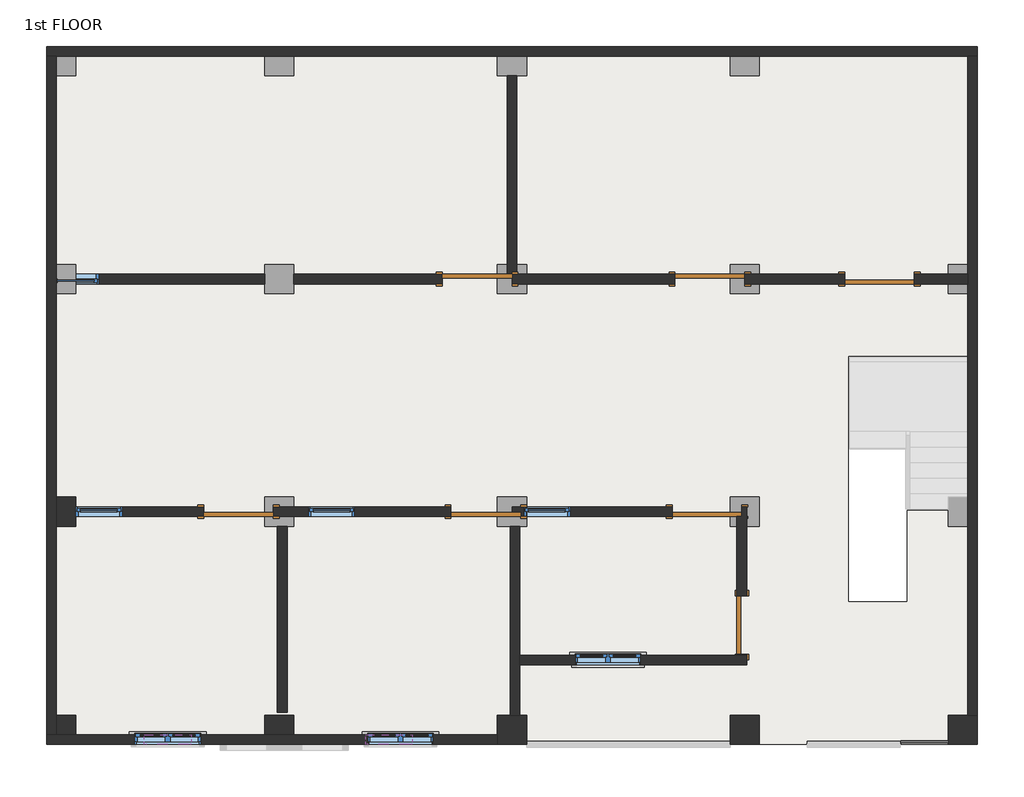
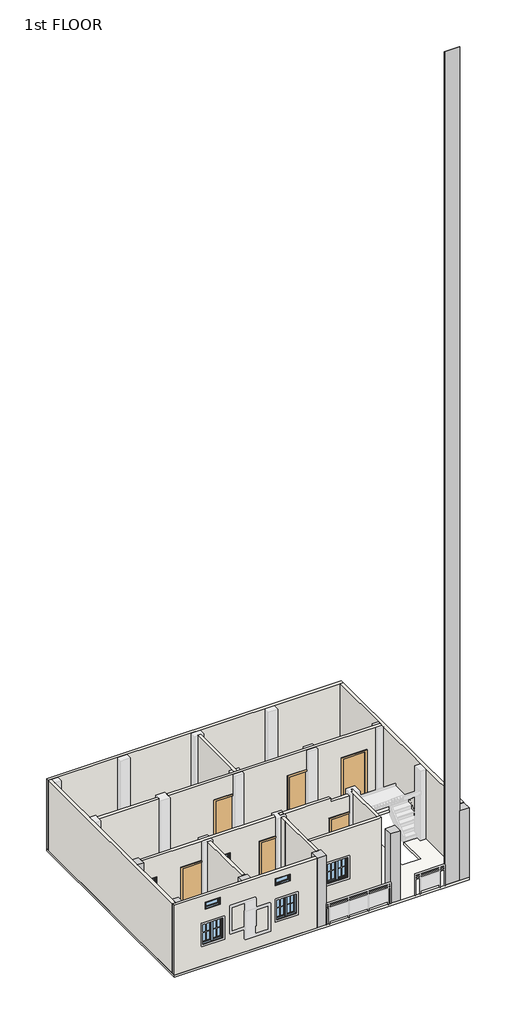
# One storey, part 1 of 2: 15 walls, 9 windows, 7 doors, 6 columns, 1 plate, 1 slab.
"""IFC4 building model written with IfcOpenShell, lengths in millimetres."""

from ifc_helpers import new_model, si_unit, frame, origin, place, context, project, spatial, polyline, outline, extrude, faceted_brep, transform, mapped, element, save
from components import door_e00f436c, door_a1797ceb, system_panel_glazed_6238d1ea, window_4c2727af, window_0bf3737e, window_78893e6c, window_0d9958e7

model = new_model("IFC4")

# Units and contexts
model_context = context("Model", 3, world=origin())
ifc_project = project(units=[si_unit("LENGTHUNIT", "METRE", prefix="MILLI")], contexts=[model_context])

# Site, building, storey
site = spatial("IfcSite", under=ifc_project)
building = spatial("IfcBuilding", under=site)
storey = spatial("IfcBuildingStorey", under=building, Name="1st FLOOR", Elevation=3048.0)

# Columns
placement = place(None, origin())
element("IfcColumn", 1, ObjectType="column family : column family", at=placement, inside=storey, context=model_context, shape_type="SweptSolid", body=[
    extrude(outline(polyline([(-15433.597125, 2867.2065522), (-15433.597125, 2486.2065522), (-15687.597125, 2486.2065522), (-15687.597125, 2867.2065522), (-15433.597125, 2867.2065522)])), frame((0.0, 0.0, 3053.0), z_axis=(0.0, 0.0, 1.0), x_axis=(1.0, 0.0, 0.0)), (0.0, 0.0, 1.0), 3038.0),
])
element("IfcColumn", 2, ObjectType="column family : column family", at=placement, inside=storey, context=model_context, shape_type="Brep", body=[
    faceted_brep([(-15433.597125, 9.7065522, 3053.0), (-15433.597125, -244.2934478, 3053.0), (-15687.597125, -244.2934478, 3053.0), (-15687.597125, 9.7065522, 3053.0), (-15433.597125, 9.7065522, 6091.0), (-15433.597125, -244.2934478, 6091.0), (-15687.597125, 9.7065522, 6091.0), (-15687.597125, -244.2934478, 6091.0), (-15687.597125, -244.2934478, 5943.6)], [[[0, 1, 2, 3]], [[0, 4, 5, 1]], [[4, 0, 3, 6]], [[5, 4, 6, 7]], [[1, 5, 7, 8, 2]], [[3, 2, 8, 7, 6]]]),
])
element("IfcColumn", 3, ObjectType="column family : column family", at=placement, inside=storey, context=model_context, shape_type="Brep", body=[
    faceted_brep([(-3622.597125, 9.7065522, 3053.0), (-3622.597125, -371.2934478, 3053.0), (-4003.597125, -371.2934478, 3053.0), (-4003.597125, 9.7065522, 3053.0), (-3622.597125, 9.7065522, 6091.0), (-3622.597125, -371.2934478, 6091.0), (-3622.597125, 9.7065522, 5943.6), (-4003.597125, -371.2934478, 6091.0), (-4003.597125, 9.7065522, 6091.0)], [[[0, 1, 2, 3]], [[4, 5, 1, 0, 6]], [[5, 7, 2, 1]], [[7, 8, 3, 2]], [[8, 4, 6, 0, 3]], [[4, 8, 7, 5]]]),
])
element("IfcColumn", 4, ObjectType="column family : column family", at=placement, inside=storey, context=model_context, shape_type="SweptSolid", body=[
    extrude(outline(polyline([(-6480.097125, 9.7065522), (-6480.097125, -371.2934478), (-6861.097125, -371.2934478), (-6861.097125, 9.7065522), (-6480.097125, 9.7065522)])), frame((0.0, 0.0, 3053.0), z_axis=(0.0, 0.0, 1.0), x_axis=(1.0, 0.0, 0.0)), (0.0, 0.0, 1.0), 3038.0),
])
element("IfcColumn", 5, ObjectType="column family : column family", at=placement, inside=storey, context=model_context, shape_type="Brep", body=[
    faceted_brep([(-9528.097125, 9.7065522, 3053.0), (-9528.097125, -371.2934478, 3053.0), (-9909.097125, -371.2934478, 3053.0), (-9909.097125, 9.7065522, 3053.0), (-9528.097125, 9.7065522, 6091.0), (-9528.097125, -371.2934478, 6091.0), (-9909.097125, -371.2934478, 6091.0), (-9909.097125, -371.2934478, 5943.6), (-9909.097125, 9.7065522, 6091.0)], [[[0, 1, 2, 3]], [[4, 5, 1, 0]], [[5, 6, 7, 2, 1]], [[6, 8, 3, 2, 7]], [[8, 4, 0, 3]], [[4, 8, 6, 5]]]),
])
element("IfcColumn", 6, ObjectType="column family : column family", at=placement, inside=storey, context=model_context, shape_type="SweptSolid", body=[
    extrude(outline(polyline([(-12957.097125, 9.7065522), (-12576.097125, 9.7065522), (-12576.097125, -244.2934478), (-12957.097125, -244.2934478), (-12957.097125, 9.7065522)])), frame((0.0, 0.0, 3053.0), z_axis=(0.0, 0.0, 1.0), x_axis=(1.0, 0.0, 0.0)), (0.0, 0.0, 1.0), 3038.0),
])

# Doors
door_shape = door_e00f436c(model_context)
element("IfcDoor", 7, ObjectType="Single-Flush : 30\" x 80\"", at=placement, inside=storey, context=model_context, shape_type="MappedRepresentation", body=[
    mapped(door_shape, transform((-6708.697125, 1190.8065522, 3048.0), x_axis=(0.0, -1.0, 0.0), y_axis=(1.0, 0.0, 0.0), z_axis=(0.0, 0.0, 1.0))),
])
door_2_shape = door_a1797ceb(model_context)
element("IfcDoor", 8, ObjectType="Single-Flush : 36\" x 84\"", at=placement, inside=storey, context=model_context, shape_type="MappedRepresentation", body=[
    mapped(door_2_shape, transform((-10175.797125, 5724.7065522, 3048.0), x_axis=(1.0, 0.0, 0.0), y_axis=(0.0, 1.0, 0.0), z_axis=(0.0, 0.0, 1.0))),
])
element("IfcDoor", 9, ObjectType="Single-Flush : 36\" x 84\"", at=placement, inside=storey, context=model_context, shape_type="MappedRepresentation", body=[
    mapped(door_2_shape, transform((-10061.497125, 2676.7065522, 3048.0), x_axis=(-1.0, 0.0, 0.0), y_axis=(0.0, -1.0, 0.0), z_axis=(0.0, 0.0, 1.0))),
])
element("IfcDoor", 10, ObjectType="Single-Flush : 36\" x 84\"", at=placement, inside=storey, context=model_context, shape_type="MappedRepresentation", body=[
    mapped(door_2_shape, transform((-13299.997125, 2676.7065522, 3048.0), x_axis=(-1.0, 0.0, 0.0), y_axis=(0.0, -1.0, 0.0), z_axis=(0.0, 0.0, 1.0))),
])
element("IfcDoor", 11, ObjectType="Single-Flush : 36\" x 84\"", at=placement, inside=storey, context=model_context, shape_type="MappedRepresentation", body=[
    mapped(door_2_shape, transform((-7127.797125, 5724.7065522, 3048.0), x_axis=(1.0, 0.0, 0.0), y_axis=(0.0, 1.0, 0.0), z_axis=(0.0, 0.0, 1.0))),
])
element("IfcDoor", 12, ObjectType="Single-Flush : 36\" x 84\"", at=placement, inside=storey, context=model_context, shape_type="MappedRepresentation", body=[
    mapped(door_2_shape, transform((-7165.897125, 2676.7065522, 3048.0), x_axis=(-1.0, 0.0, 0.0), y_axis=(0.0, -1.0, 0.0), z_axis=(0.0, 0.0, 1.0))),
])
element("IfcDoor", 13, ObjectType="Single-Flush : 36\" x 84\"", at=placement, inside=storey, context=model_context, shape_type="MappedRepresentation", body=[
    mapped(door_2_shape, transform((-4905.297125, 5724.7065522, 3048.0), x_axis=(-1.0, 0.0, 0.0), y_axis=(0.0, -1.0, 0.0), z_axis=(0.0, 0.0, 1.0))),
])

# Plate
system_panel_glazed_shape = system_panel_glazed_6238d1ea(model_context)
element("IfcPlate", 14, ObjectType="System Panel : Glazed", at=placement, inside=storey, context=model_context, shape_type="MappedRepresentation", body=[
    mapped(system_panel_glazed_shape, transform((-4314.747125, -371.2934478, 3048.0), x_axis=(1.0, 0.0, 0.0), y_axis=(0.0, 1.0, 0.0), z_axis=(0.0, 0.0, 1.0))),
])

# Slab
element("IfcSlab", 15, ObjectType="Generic - 4\"", at=placement, inside=storey, context=model_context, shape_type="SweptSolid", body=[
    extrude(outline(polyline([(-3622.597125, 8772.7065522), (-3622.597125, -371.2934478), (-15814.597125, -371.2934478), (-15814.597125, 8772.7065522), (-3622.597125, 8772.7065522)]), holes=[polyline([(-3734.357125, 4711.0719226), (-5310.2646464, 4711.0719226), (-5310.2646464, 1502.3126957), (-4547.7736682, 1502.3126957), (-4547.7736682, 2699.911213), (-3734.357125, 2699.911213), (-3734.357125, 4711.0719226)])]), frame((0.0, 0.0, 2946.4), z_axis=(0.0, 0.0, 1.0), x_axis=(1.0, 0.0, 0.0)), (0.0, 0.0, 1.0), 101.6),
])

# Walls
element("IfcWall", 16, ObjectType="Generic - 5\"", at=placement, inside=storey, context=model_context, shape_type="Brep", body=[
    faceted_brep([(-15814.597125, 8645.7065522, 6096.0), (-15814.597125, 8645.7065522, 5943.6), (-15814.597125, 8645.7065522, 3048.0), (-15687.597125, 8645.7065522, 3048.0), (-3749.597125, 8645.7065522, 3048.0), (-3622.597125, 8645.7065522, 3048.0), (-3622.597125, 8645.7065522, 5943.6), (-3622.597125, 8645.7065522, 6096.0), (-3749.597125, 8645.7065522, 6096.0), (-15687.597125, 8645.7065522, 6096.0), (-15814.597125, 8772.7065522, 3048.0), (-15814.597125, 8772.7065522, 6096.0), (-15687.597125, 8772.7065522, 6096.0), (-3749.597125, 8772.7065522, 6096.0), (-3622.597125, 8772.7065522, 6096.0), (-3622.597125, 8772.7065522, 3048.0)], [[[0, 1, 2, 3, 4, 5, 6, 7, 8, 9]], [[10, 11, 12, 13, 14, 15]], [[5, 4, 3, 2, 10, 15]], [[0, 9, 8, 7, 14, 13, 12, 11]], [[5, 15, 14, 7, 6]], [[0, 11, 10, 2, 1]]]),
])
element("IfcWall", 17, ObjectType="Generic - 5\"", at=placement, inside=storey, context=model_context, shape_type="Brep", body=[
    faceted_brep([(-3749.597125, 8645.7065522, 6096.0), (-3749.597125, 8645.7065522, 3048.0), (-3749.597125, 5788.2065522, 3048.0), (-3749.597125, 5661.2065522, 3048.0), (-3749.597125, 9.7065522, 3048.0), (-3749.597125, 9.7065522, 6096.0), (-3749.597125, 5661.2065522, 6096.0), (-3749.597125, 5788.2065522, 6096.0), (-3622.597125, 8645.7065522, 3048.0), (-3622.597125, 8645.7065522, 6096.0), (-3622.597125, 9.7065522, 6096.0), (-3622.597125, 9.7065522, 6091.0), (-3622.597125, 9.7065522, 5948.6), (-3622.597125, 9.7065522, 3053.0), (-3622.597125, 9.7065522, 3048.0)], [[[0, 1, 2, 3, 4, 5, 6, 7]], [[8, 9, 10, 11, 12, 13, 14]], [[4, 3, 2, 1, 8, 14]], [[5, 4, 14, 13, 12, 11, 10]], [[0, 7, 6, 5, 10, 9]], [[0, 9, 8, 1]]]),
])
element("IfcWall", 18, ObjectType="Generic - 5\"", at=placement, inside=storey, context=model_context, shape_type="Brep", body=[
    faceted_brep([(-9909.097125, -244.2934478, 3048.0), (-15687.597125, -244.2934478, 3048.0), (-15814.597125, -244.2934478, 3048.0), (-15814.597125, -244.2934478, 5943.6), (-15814.597125, -244.2934478, 6096.0), (-15687.597125, -244.2934478, 6096.0), (-9909.097125, -244.2934478, 6096.0), (-13795.297125, -244.2934478, 4876.8), (-14658.897125, -244.2934478, 4876.8), (-14658.897125, -244.2934478, 3962.4), (-13795.297125, -244.2934478, 3962.4), (-10747.297125, -244.2934478, 4876.8), (-11610.897125, -244.2934478, 4876.8), (-11610.897125, -244.2934478, 3962.4), (-10747.297125, -244.2934478, 3962.4), (-13922.297125, -244.2934478, 5791.2), (-14531.897125, -244.2934478, 5791.2), (-14531.897125, -244.2934478, 5486.4), (-13922.297125, -244.2934478, 5486.4), (-11026.697125, -244.2934478, 5791.2), (-11636.297125, -244.2934478, 5791.2), (-11636.297125, -244.2934478, 5486.4), (-11026.697125, -244.2934478, 5486.4), (-9909.097125, -371.2934478, 3048.0), (-9909.097125, -371.2934478, 3053.0), (-9909.097125, -371.2934478, 5948.6), (-9909.097125, -371.2934478, 6091.0), (-9909.097125, -371.2934478, 6096.0), (-15687.597125, -371.2934478, 6096.0), (-15814.597125, -371.2934478, 6096.0), (-15814.597125, -371.2934478, 3048.0), (-13795.297125, -371.2934478, 4876.8), (-13795.297125, -371.2934478, 3962.4), (-14658.897125, -371.2934478, 3962.4), (-14658.897125, -371.2934478, 4876.8), (-10747.297125, -371.2934478, 4876.8), (-10747.297125, -371.2934478, 3962.4), (-11610.897125, -371.2934478, 3962.4), (-11610.897125, -371.2934478, 4876.8), (-13922.297125, -371.2934478, 5791.2), (-13922.297125, -371.2934478, 5486.4), (-14531.897125, -371.2934478, 5486.4), (-14531.897125, -371.2934478, 5791.2), (-11026.697125, -371.2934478, 5791.2), (-11026.697125, -371.2934478, 5486.4), (-11636.297125, -371.2934478, 5486.4), (-11636.297125, -371.2934478, 5791.2)], [[[0, 1, 2, 3, 4, 5, 6], [7, 8, 9, 10], [11, 12, 13, 14], [15, 16, 17, 18], [19, 20, 21, 22]], [[23, 24, 25, 26, 27, 28, 29, 30], [31, 32, 33, 34], [35, 36, 37, 38], [39, 40, 41, 42], [43, 44, 45, 46]], [[2, 1, 0, 23, 30]], [[6, 5, 4, 29, 28, 27]], [[0, 6, 27, 26, 25, 24, 23]], [[32, 31, 7, 10]], [[33, 32, 10, 9]], [[34, 33, 9, 8]], [[31, 34, 8, 7]], [[36, 35, 11, 14]], [[37, 36, 14, 13]], [[38, 37, 13, 12]], [[35, 38, 12, 11]], [[40, 39, 15, 18]], [[41, 40, 18, 17]], [[42, 41, 17, 16]], [[39, 42, 16, 15]], [[44, 43, 19, 22]], [[45, 44, 22, 21]], [[46, 45, 21, 20]], [[43, 46, 20, 19]], [[2, 30, 29, 4, 3]]]),
])
element("IfcWall", 19, ObjectType="Generic - 5\"", at=placement, inside=storey, context=model_context, shape_type="Brep", body=[
    faceted_brep([(-15687.597125, -244.2934478, 6096.0), (-15687.597125, -244.2934478, 6091.0), (-15687.597125, -244.2934478, 5948.6), (-15687.597125, -244.2934478, 3053.0), (-15687.597125, -244.2934478, 3048.0), (-15687.597125, 8645.7065522, 3048.0), (-15687.597125, 8645.7065522, 3053.0), (-15687.597125, 8645.7065522, 5948.6), (-15687.597125, 8645.7065522, 6091.0), (-15687.597125, 8645.7065522, 6096.0), (-15814.597125, -244.2934478, 3048.0), (-15814.597125, -244.2934478, 6096.0), (-15814.597125, 8645.7065522, 6096.0), (-15814.597125, 8645.7065522, 3048.0)], [[[0, 1, 2, 3, 4, 5, 6, 7, 8, 9]], [[10, 11, 12, 13]], [[5, 4, 10, 13]], [[0, 9, 12, 11]], [[5, 13, 12, 9, 8, 7, 6]], [[0, 11, 10, 4, 3, 2, 1]]]),
])
element("IfcWall", 20, ObjectType="Generic - 5\"", at=placement, inside=storey, context=model_context, shape_type="SweptSolid", body=[
    extrude(outline(polyline([(3048.0, -15433.597125), (3048.0, -12957.097125), (6096.0, -12957.097125), (6096.0, -15433.597125), (5181.6, -15433.597125), (5181.6, -15128.797125), (3352.8, -15128.797125), (3352.8, -15433.597125), (3048.0, -15433.597125)])), frame((0.0, 5661.2065522, 0.0), z_axis=(0.0, 1.0, 0.0), x_axis=(0.0, 0.0, 1.0)), (0.0, 0.0, 1.0), 127.0),
])
element("IfcWall", 21, ObjectType="Generic - 5\"", at=placement, inside=storey, context=model_context, shape_type="Brep", body=[
    faceted_brep([(-9782.097125, 8391.7065522, 3048.0), (-9782.097125, 5788.2065522, 3048.0), (-9782.097125, 5788.2065522, 3053.0), (-9782.097125, 5788.2065522, 5181.6), (-9782.097125, 5788.2065522, 5948.6), (-9782.097125, 5788.2065522, 6091.0), (-9782.097125, 5788.2065522, 6096.0), (-9782.097125, 8391.7065522, 6096.0), (-9655.097125, 8391.7065522, 3048.0), (-9655.097125, 8391.7065522, 6096.0), (-9655.097125, 5788.2065522, 6096.0), (-9655.097125, 5788.2065522, 6091.0), (-9655.097125, 5788.2065522, 5948.6), (-9655.097125, 5788.2065522, 3053.0), (-9655.097125, 5788.2065522, 3048.0), (-9718.597125, 5788.2065522, 3048.0)], [[[0, 1, 2, 3, 4, 5, 6, 7]], [[8, 9, 10, 11, 12, 13, 14]], [[1, 0, 8, 14, 15]], [[7, 6, 10, 9]], [[0, 7, 9, 8]], [[6, 5, 4, 3, 2, 1, 15, 14, 13, 12, 11, 10]]]),
])
element("IfcWall", 22, ObjectType="Generic - 5\"", at=placement, inside=storey, context=model_context, shape_type="Brep", body=[
    faceted_brep([(-6670.597125, 5661.2065522, 3048.0), (-5362.497125, 5661.2065522, 3048.0), (-5362.497125, 5661.2065522, 5181.6), (-4448.097125, 5661.2065522, 5181.6), (-4448.097125, 5661.2065522, 3048.0), (-3749.597125, 5661.2065522, 3048.0), (-3749.597125, 5661.2065522, 3053.0), (-3749.597125, 5661.2065522, 5948.6), (-3749.597125, 5661.2065522, 6091.0), (-3749.597125, 5661.2065522, 6096.0), (-6670.597125, 5661.2065522, 6096.0), (-6861.097125, 5661.2065522, 6096.0), (-9718.597125, 5661.2065522, 6096.0), (-9909.097125, 5661.2065522, 6096.0), (-12576.097125, 5661.2065522, 6096.0), (-12576.097125, 5661.2065522, 3048.0), (-10632.997125, 5661.2065522, 3048.0), (-10632.997125, 5661.2065522, 5181.6), (-9909.097125, 5661.2065522, 5181.6), (-9718.597125, 5661.2065522, 5181.6), (-9718.597125, 5661.2065522, 3053.0), (-9718.597125, 5661.2065522, 3048.0), (-7584.997125, 5661.2065522, 3048.0), (-7584.997125, 5661.2065522, 5181.6), (-6861.097125, 5661.2065522, 5181.6), (-6670.597125, 5661.2065522, 5181.6), (-6670.597125, 5661.2065522, 3053.0), (-5362.497125, 5788.2065522, 5181.6), (-5362.497125, 5788.2065522, 3048.0), (-6670.597125, 5788.2065522, 3048.0), (-6670.597125, 5788.2065522, 3053.0), (-6670.597125, 5788.2065522, 5181.6), (-6861.097125, 5788.2065522, 5181.6), (-7584.997125, 5788.2065522, 5181.6), (-7584.997125, 5788.2065522, 3048.0), (-9655.097125, 5788.2065522, 3048.0), (-9718.597125, 5788.2065522, 3048.0), (-9718.597125, 5788.2065522, 3053.0), (-9718.597125, 5788.2065522, 5181.6), (-9782.097125, 5788.2065522, 5181.6), (-9909.097125, 5788.2065522, 5181.6), (-10632.997125, 5788.2065522, 5181.6), (-10632.997125, 5788.2065522, 3048.0), (-12576.097125, 5788.2065522, 3048.0), (-12576.097125, 5788.2065522, 6096.0), (-9909.097125, 5788.2065522, 6096.0), (-9782.097125, 5788.2065522, 6096.0), (-9718.597125, 5788.2065522, 6096.0), (-9655.097125, 5788.2065522, 6096.0), (-6861.097125, 5788.2065522, 6096.0), (-6670.597125, 5788.2065522, 6096.0), (-3749.597125, 5788.2065522, 6096.0), (-3749.597125, 5788.2065522, 6091.0), (-3749.597125, 5788.2065522, 5948.6), (-3749.597125, 5788.2065522, 3053.0), (-3749.597125, 5788.2065522, 3048.0), (-4448.097125, 5788.2065522, 3048.0), (-4448.097125, 5788.2065522, 5181.6)], [[[0, 1, 2, 3, 4, 5, 6, 7, 8, 9, 10, 11, 12, 13, 14, 15, 16, 17, 18, 19, 20, 21, 22, 23, 24, 25, 26]], [[27, 28, 29, 30, 31, 32, 33, 34, 35, 36, 37, 38, 39, 40, 41, 42, 43, 44, 45, 46, 47, 48, 49, 50, 51, 52, 53, 54, 55, 56, 57]], [[16, 15, 43, 42]], [[22, 21, 36, 35, 34]], [[56, 55, 5, 4]], [[29, 28, 1, 0]], [[14, 13, 12, 11, 10, 9, 51, 50, 49, 48, 47, 46, 45, 44]], [[15, 14, 44, 43]], [[9, 8, 7, 6, 5, 55, 54, 53, 52, 51]], [[38, 37, 36, 21, 20, 19]], [[41, 40, 39, 38, 19, 18, 17]], [[42, 41, 17, 16]], [[31, 30, 29, 0, 26, 25]], [[33, 32, 31, 25, 24, 23]], [[34, 33, 23, 22]], [[2, 1, 28, 27]], [[3, 2, 27, 57]], [[4, 3, 57, 56]]]),
])
element("IfcWall", 23, ObjectType="Generic - 5\"", at=placement, inside=storey, context=model_context, shape_type="Brep", body=[
    faceted_brep([(-14823.997125, 2613.2065522, 3352.8), (-15433.597125, 2613.2065522, 3352.8), (-15433.597125, 2613.2065522, 3048.0), (-13757.197125, 2613.2065522, 3048.0), (-13757.197125, 2613.2065522, 5181.6), (-12957.097125, 2613.2065522, 5181.6), (-12842.797125, 2613.2065522, 5181.6), (-12842.797125, 2613.2065522, 3053.0), (-12842.797125, 2613.2065522, 3048.0), (-10518.697125, 2613.2065522, 3048.0), (-10518.697125, 2613.2065522, 5181.6), (-9909.097125, 2613.2065522, 5181.6), (-9909.097125, 2613.2065522, 6096.0), (-12842.797125, 2613.2065522, 6096.0), (-12957.097125, 2613.2065522, 6096.0), (-15433.597125, 2613.2065522, 6096.0), (-15433.597125, 2613.2065522, 5181.6), (-14823.997125, 2613.2065522, 5181.6), (-12385.597125, 2613.2065522, 5181.6), (-11775.997125, 2613.2065522, 5181.6), (-11775.997125, 2613.2065522, 3352.8), (-12385.597125, 2613.2065522, 3352.8), (-15433.597125, 2740.2065522, 3048.0), (-15433.597125, 2740.2065522, 3352.8), (-14823.997125, 2740.2065522, 3352.8), (-14823.997125, 2740.2065522, 5181.6), (-15433.597125, 2740.2065522, 5181.6), (-15433.597125, 2740.2065522, 6096.0), (-12957.097125, 2740.2065522, 6096.0), (-12842.797125, 2740.2065522, 6096.0), (-9909.097125, 2740.2065522, 6096.0), (-9909.097125, 2740.2065522, 5181.6), (-10518.697125, 2740.2065522, 5181.6), (-10518.697125, 2740.2065522, 3048.0), (-12842.797125, 2740.2065522, 3048.0), (-12842.797125, 2740.2065522, 3053.0), (-12842.797125, 2740.2065522, 5181.6), (-12957.097125, 2740.2065522, 5181.6), (-13757.197125, 2740.2065522, 5181.6), (-13757.197125, 2740.2065522, 3048.0), (-12385.597125, 2740.2065522, 5181.6), (-12385.597125, 2740.2065522, 3352.8), (-11775.997125, 2740.2065522, 3352.8), (-11775.997125, 2740.2065522, 5181.6)], [[[0, 1, 2, 3, 4, 5, 6, 7, 8, 9, 10, 11, 12, 13, 14, 15, 16, 17], [18, 19, 20, 21]], [[22, 23, 24, 25, 26, 27, 28, 29, 30, 31, 32, 33, 34, 35, 36, 37, 38, 39], [40, 41, 42, 43]], [[34, 33, 9, 8]], [[22, 39, 3, 2]], [[30, 12, 11, 31]], [[15, 14, 13, 12, 30, 29, 28, 27]], [[16, 15, 27, 26]], [[2, 1, 23, 22]], [[32, 10, 9, 33]], [[10, 32, 31, 11]], [[4, 3, 39, 38]], [[6, 5, 4, 38, 37, 36]], [[8, 7, 6, 36, 35, 34]], [[24, 23, 1, 0]], [[25, 24, 0, 17]], [[26, 25, 17, 16]], [[41, 40, 18, 21]], [[42, 41, 21, 20]], [[43, 42, 20, 19]], [[40, 43, 19, 18]]]),
])
element("IfcWall", 24, ObjectType="Generic - 5\"", at=placement, inside=storey, context=model_context, shape_type="Brep", body=[
    faceted_brep([(-9616.997125, 9.7065522, 3048.0), (-9616.997125, 670.1065522, 3048.0), (-9616.997125, 797.1065522, 3048.0), (-9616.997125, 2486.2065522, 3048.0), (-9616.997125, 2486.2065522, 6096.0), (-9616.997125, 797.1065522, 6096.0), (-9616.997125, 670.1065522, 6096.0), (-9616.997125, 9.7065522, 6096.0), (-9743.997125, 9.7065522, 3048.0), (-9743.997125, 9.7065522, 6096.0), (-9743.997125, 2486.2065522, 6096.0), (-9743.997125, 2486.2065522, 3048.0)], [[[0, 1, 2, 3, 4, 5, 6, 7]], [[8, 9, 10, 11]], [[3, 2, 1, 0, 8, 11]], [[4, 3, 11, 10]], [[7, 6, 5, 4, 10, 9]], [[0, 7, 9, 8]]]),
])
element("IfcWall", 25, ObjectType="Generic - 5\"", at=placement, inside=storey, context=model_context, shape_type="SweptSolid", body=[
    extrude(outline(polyline([(-9743.997125, 2181.4065522), (-9743.997125, 2486.2065522), (-9616.997125, 2486.2065522), (-9616.997125, 2181.4065522), (-9743.997125, 2181.4065522)])), frame((0.0, 0.0, 3048.0), z_axis=(0.0, 0.0, 1.0), x_axis=(1.0, 0.0, 0.0)), (0.0, 0.0, 1.0), 3048.0),
])
element("IfcWall", 26, ObjectType="Generic - 5\"", at=placement, inside=storey, context=model_context, shape_type="Brep", body=[
    faceted_brep([(-9718.597125, 2613.2065522, 6096.0), (-9718.597125, 2613.2065522, 6091.0), (-9718.597125, 2613.2065522, 5948.6), (-9718.597125, 2613.2065522, 3053.0), (-9718.597125, 2613.2065522, 3048.0), (-7623.097125, 2613.2065522, 3048.0), (-7623.097125, 2613.2065522, 5181.6), (-6861.097125, 2613.2065522, 5181.6), (-6772.197125, 2613.2065522, 5181.6), (-6772.197125, 2613.2065522, 5943.6), (-6861.097125, 2613.2065522, 5943.6), (-7623.097125, 2613.2065522, 5943.6), (-7623.097125, 2613.2065522, 6096.0), (-9566.197125, 2613.2065522, 5181.6), (-9528.097125, 2613.2065522, 5181.6), (-8956.597125, 2613.2065522, 5181.6), (-8956.597125, 2613.2065522, 3352.8), (-9528.097125, 2613.2065522, 3352.8), (-9566.197125, 2613.2065522, 3352.8), (-9718.597125, 2740.2065522, 3048.0), (-9718.597125, 2740.2065522, 3053.0), (-9718.597125, 2740.2065522, 5948.6), (-9718.597125, 2740.2065522, 6091.0), (-9718.597125, 2740.2065522, 6096.0), (-7623.097125, 2740.2065522, 6096.0), (-7623.097125, 2740.2065522, 5943.6), (-6861.097125, 2740.2065522, 5943.6), (-6772.197125, 2740.2065522, 5943.6), (-6772.197125, 2740.2065522, 5181.6), (-6861.097125, 2740.2065522, 5181.6), (-7623.097125, 2740.2065522, 5181.6), (-7623.097125, 2740.2065522, 3048.0), (-9566.197125, 2740.2065522, 5181.6), (-9566.197125, 2740.2065522, 3352.8), (-9528.097125, 2740.2065522, 3352.8), (-8956.597125, 2740.2065522, 3352.8), (-8956.597125, 2740.2065522, 5181.6), (-9528.097125, 2740.2065522, 5181.6)], [[[0, 1, 2, 3, 4, 5, 6, 7, 8, 9, 10, 11, 12], [13, 14, 15, 16, 17, 18]], [[19, 20, 21, 22, 23, 24, 25, 26, 27, 28, 29, 30, 31], [32, 33, 34, 35, 36, 37]], [[4, 19, 31, 5]], [[23, 0, 12, 24]], [[4, 3, 2, 1, 0, 23, 22, 21, 20, 19]], [[33, 32, 13, 18]], [[35, 34, 33, 18, 17, 16]], [[36, 35, 16, 15]], [[32, 37, 36, 15, 14, 13]], [[30, 6, 5, 31]], [[6, 30, 29, 28, 8, 7]], [[8, 28, 27, 9]], [[25, 11, 10, 9, 27, 26]], [[11, 25, 24, 12]]]),
])
element("IfcWall", 27, ObjectType="Generic - 5\"", at=placement, inside=storey, context=model_context, shape_type="Brep", body=[
    faceted_brep([(-6645.197125, 2740.2065522, 6096.0), (-6645.197125, 2613.2065522, 6096.0), (-6645.197125, 797.1065522, 6096.0), (-6645.197125, 797.1065522, 3048.0), (-6645.197125, 809.8065522, 3048.0), (-6645.197125, 809.8065522, 5080.0), (-6645.197125, 1571.8065522, 5080.0), (-6645.197125, 1571.8065522, 3048.0), (-6645.197125, 2740.2065522, 3048.0), (-6645.197125, 2740.2065522, 3053.0), (-6645.197125, 2740.2065522, 5948.6), (-6645.197125, 2740.2065522, 6091.0), (-6772.197125, 2613.2065522, 5181.6), (-6772.197125, 2613.2065522, 3053.0), (-6772.197125, 2613.2065522, 3048.0), (-6772.197125, 1571.8065522, 3048.0), (-6772.197125, 1571.8065522, 5080.0), (-6772.197125, 809.8065522, 5080.0), (-6772.197125, 809.8065522, 3048.0), (-6772.197125, 797.1065522, 3048.0), (-6772.197125, 797.1065522, 6096.0), (-6772.197125, 2613.2065522, 6096.0), (-6772.197125, 2613.2065522, 6091.0), (-6772.197125, 2613.2065522, 5948.6), (-6772.197125, 2613.2065522, 5943.6), (-6772.197125, 2740.2065522, 5943.6), (-6772.197125, 2740.2065522, 5181.6), (-6708.697125, 2613.2065522, 3048.0), (-6708.697125, 2740.2065522, 3048.0), (-6708.697125, 2740.2065522, 6096.0), (-6708.697125, 2613.2065522, 6096.0), (-6708.697125, 2613.2065522, 5181.6), (-6708.697125, 2613.2065522, 3053.0), (-6708.697125, 2740.2065522, 5181.6), (-6708.697125, 2740.2065522, 3053.0), (-6708.697125, 2740.2065522, 5943.6), (-6708.697125, 2740.2065522, 5948.6), (-6708.697125, 2740.2065522, 6091.0), (-6708.697125, 2613.2065522, 5943.6), (-6708.697125, 2613.2065522, 6091.0), (-6708.697125, 2613.2065522, 5948.6)], [[[0, 1, 2, 3, 4, 5, 6, 7, 8, 9, 10, 11]], [[12, 13, 14, 15, 16, 17, 18, 19, 20, 21, 22, 23, 24, 25, 26]], [[14, 27, 28, 8, 7, 15]], [[3, 19, 18, 4]], [[2, 1, 0, 29, 30, 21, 20]], [[31, 32, 27, 14, 13, 12]], [[33, 31, 12, 26]], [[27, 32, 31, 33, 34, 28]], [[5, 4, 18, 17]], [[6, 5, 17, 16]], [[7, 6, 16, 15]], [[8, 28, 34, 33, 26, 25, 35, 36, 37, 29, 0, 11, 10, 9]], [[2, 20, 19, 3]], [[38, 24, 23, 22, 21, 30, 39, 40]], [[38, 35, 25, 24]], [[35, 38, 40, 39, 30, 29, 37, 36]]]),
])
element("IfcWall", 28, ObjectType="Generic - 5\"", at=placement, inside=storey, context=model_context, shape_type="Brep", body=[
    faceted_brep([(-9718.597125, 2613.2065522, 3048.0), (-9566.197125, 2613.2065522, 3048.0), (-9566.197125, 2613.2065522, 3352.8), (-9566.197125, 2613.2065522, 5181.6), (-9566.197125, 2613.2065522, 6096.0), (-9718.597125, 2613.2065522, 6096.0), (-9718.597125, 2613.2065522, 6091.0), (-9718.597125, 2613.2065522, 5948.6), (-9718.597125, 2613.2065522, 3053.0), (-9718.597125, 2740.2065522, 3048.0), (-9718.597125, 2740.2065522, 3053.0), (-9718.597125, 2740.2065522, 5948.6), (-9718.597125, 2740.2065522, 6091.0), (-9718.597125, 2740.2065522, 6096.0), (-9566.197125, 2740.2065522, 6096.0), (-9566.197125, 2740.2065522, 5181.6), (-9566.197125, 2740.2065522, 3352.8), (-9566.197125, 2740.2065522, 3048.0)], [[[0, 1, 2, 3, 4, 5, 6, 7, 8]], [[9, 10, 11, 12, 13, 14, 15, 16, 17]], [[1, 0, 9, 17]], [[4, 3, 2, 1, 17, 16, 15, 14]], [[5, 4, 14, 13]], [[0, 8, 7, 6, 5, 13, 12, 11, 10, 9]]]),
])
element("IfcWall", 29, ObjectType="Generic - 5\"", at=placement, inside=storey, context=model_context, shape_type="SweptSolid", body=[
    extrude(outline(polyline([(-12791.997125, 47.8065522), (-12791.997125, 2486.2065522), (-12664.997125, 2486.2065522), (-12664.997125, 47.8065522), (-12791.997125, 47.8065522)])), frame((0.0, 0.0, 3048.0), z_axis=(0.0, 0.0, 1.0), x_axis=(1.0, 0.0, 0.0)), (0.0, 0.0, 1.0), 3048.0),
])
element("IfcWall", 30, ObjectType="Generic - 5\"", at=placement, inside=storey, context=model_context, shape_type="Brep", body=[
    faceted_brep([(-9616.997125, 670.1065522, 3048.0), (-6645.197125, 670.1065522, 3048.0), (-6645.197125, 670.1065522, 6096.0), (-6772.197125, 670.1065522, 6096.0), (-9616.997125, 670.1065522, 6096.0), (-8029.497125, 670.1065522, 4876.8), (-8029.497125, 670.1065522, 3962.4), (-8893.097125, 670.1065522, 3962.4), (-8893.097125, 670.1065522, 4876.8), (-9616.997125, 797.1065522, 3048.0), (-9616.997125, 797.1065522, 6096.0), (-6772.197125, 797.1065522, 6096.0), (-6645.197125, 797.1065522, 6096.0), (-6645.197125, 797.1065522, 5943.6), (-6645.197125, 797.1065522, 3048.0), (-6772.197125, 797.1065522, 3048.0), (-8029.497125, 797.1065522, 4876.8), (-8893.097125, 797.1065522, 4876.8), (-8893.097125, 797.1065522, 3962.4), (-8029.497125, 797.1065522, 3962.4)], [[[0, 1, 2, 3, 4], [5, 6, 7, 8]], [[9, 10, 11, 12, 13, 14, 15], [16, 17, 18, 19]], [[1, 0, 9, 15, 14]], [[4, 3, 2, 12, 11, 10]], [[0, 4, 10, 9]], [[6, 5, 16, 19]], [[7, 6, 19, 18]], [[8, 7, 18, 17]], [[5, 8, 17, 16]], [[1, 14, 13, 12, 2]]]),
])

# Windows
window_shape = window_4c2727af(model_context)
element("IfcWindow", 31, ObjectType="Fixed : 24\" x 12\"", at=placement, inside=storey, context=model_context, shape_type="MappedRepresentation", body=[
    mapped(window_shape, transform((-14188.997125, -307.7934478, 4572.0), x_axis=(1.0, 0.0, 0.0), y_axis=(0.0, 1.0, 0.0), z_axis=(0.0, 0.0, 1.0))),
])
element("IfcWindow", 32, ObjectType="Fixed : 24\" x 12\"", at=placement, inside=storey, context=model_context, shape_type="MappedRepresentation", body=[
    mapped(window_shape, transform((-11293.397125, -307.7934478, 4572.0), x_axis=(1.0, 0.0, 0.0), y_axis=(0.0, 1.0, 0.0), z_axis=(0.0, 0.0, 1.0))),
])
window_2_shape = window_0bf3737e(model_context)
element("IfcWindow", 33, ObjectType="Fixed : 24\" x 72\"", at=placement, inside=storey, context=model_context, shape_type="MappedRepresentation", body=[
    mapped(window_2_shape, transform((-15471.697125, 5724.7065522, 3048.0), x_axis=(-1.0, 0.0, 0.0), y_axis=(0.0, -1.0, 0.0), z_axis=(0.0, 0.0, 1.0))),
])
window_3_shape = window_78893e6c(model_context)
element("IfcWindow", 34, ObjectType="Fixed : 24\" x 72\"", at=placement, inside=storey, context=model_context, shape_type="MappedRepresentation", body=[
    mapped(window_3_shape, transform((-15166.897125, 2676.7065522, 3048.0), x_axis=(-1.0, 0.0, 0.0), y_axis=(0.0, -1.0, 0.0), z_axis=(0.0, 0.0, 1.0))),
])
element("IfcWindow", 35, ObjectType="Fixed : 24\" x 72\"", at=placement, inside=storey, context=model_context, shape_type="MappedRepresentation", body=[
    mapped(window_3_shape, transform((-12118.897125, 2676.7065522, 3048.0), x_axis=(-1.0, 0.0, 0.0), y_axis=(0.0, -1.0, 0.0), z_axis=(0.0, 0.0, 1.0))),
])
element("IfcWindow", 36, ObjectType="Fixed : 24\" x 72\"", at=placement, inside=storey, context=model_context, shape_type="MappedRepresentation", body=[
    mapped(window_3_shape, transform((-9299.497125, 2676.7065522, 3048.0), x_axis=(-1.0, 0.0, 0.0), y_axis=(0.0, -1.0, 0.0), z_axis=(0.0, 0.0, 1.0))),
])
window_4_shape = window_0d9958e7(model_context)
element("IfcWindow", 37, ObjectType="Window-Casement-Double : 34\" x 36\"", at=placement, inside=storey, context=model_context, shape_type="MappedRepresentation", body=[
    mapped(window_4_shape, transform((-14227.097125, -307.7934478, 3048.0), x_axis=(1.0, 0.0, 0.0), y_axis=(0.0, 1.0, 0.0), z_axis=(0.0, 0.0, 1.0))),
])
element("IfcWindow", 38, ObjectType="Window-Casement-Double : 34\" x 36\"", at=placement, inside=storey, context=model_context, shape_type="MappedRepresentation", body=[
    mapped(window_4_shape, transform((-11179.097125, -307.7934478, 3048.0), x_axis=(1.0, 0.0, 0.0), y_axis=(0.0, 1.0, 0.0), z_axis=(0.0, 0.0, 1.0))),
])
element("IfcWindow", 39, ObjectType="Window-Casement-Double : 34\" x 36\"", at=placement, inside=storey, context=model_context, shape_type="MappedRepresentation", body=[
    mapped(window_4_shape, transform((-8461.297125, 733.6065522, 3048.0), x_axis=(1.0, 0.0, 0.0), y_axis=(0.0, 1.0, 0.0), z_axis=(0.0, 0.0, 1.0))),
])

save(model, "model.ifc")

# Revit data of these elements
# Type "column family : column family"
#   w2 [instance default] = 0' - 9.88189"
#   w1 [instance default] = 0' - 9.01575"
#   Depth = 1' - 11.62205"
#   Width = 1' - 11.62205"
# Type "Single-Flush : 30\" x 80\""
#   Type Mark = "5"
#   Construction Type Id = "MDOOR"
#   Assembly Code = "C1020"
#   Analytic Construction = "Metal"
#   Thickness = 0' - 2"
#   Heat Transfer Coefficient (U) = 0.651978 BTU/(h·ft²·°F)
#   Height = 6' - 8"
#   Trim Projection Ext = 0' - 1"
#   Trim Projection Int = 0' - 1"
#   Trim Width = 0' - 3"
#   Width = 2' - 6"
#   Define Thermal Properties by = 1
#   Define Thermal Properties by = 1
#   Door Material = Door - Panel
#   Frame Material = Door - Frame
#   Visual Light Transmittance = 0
#   Solar Heat Gain Coefficient = 0
#   Function = (empty or 0)
#   Wall Closure = (empty or 0)
# Type "Single-Flush : 36\" x 84\""
#   Type Mark = "1"
#   Construction Type Id = "MDOOR"
#   Assembly Code = "C1020"
#   Analytic Construction = "Metal"
#   Thickness = 0' - 2"
#   Heat Transfer Coefficient (U) = 0.651978 BTU/(h·ft²·°F)
#   Height = 7' - 0"
#   Trim Projection Ext = 0' - 1"
#   Trim Projection Int = 0' - 1"
#   Trim Width = 0' - 3"
#   Width = 3' - 0"
#   Define Thermal Properties by = 1
#   Define Thermal Properties by = 1
#   Door Material = Door - Panel
#   Frame Material = Door - Frame
#   Visual Light Transmittance = 0
#   Solar Heat Gain Coefficient = 0
#   Function = (empty or 0)
#   Wall Closure = (empty or 0)
# Type "System Panel : Glazed"
#   Construction Type Id = "GSP4R"
#   Analytic Construction = "1/8 in Pilkington single glazing"
#   Visual Light Transmittance = 0.9
#   Solar Heat Gain Coefficient = 0.86
#   Heat Transfer Coefficient (U) = 1.18115 BTU/(h·ft²·°F)
#   Define Thermal Properties by = 1
# Type "Generic - 4\""
#   Assembly Code = "B1010"
#   Function = 0
#   Layers, outside or top first: 0' - 4" no material (function 1)
# Type "Generic - 5\""
#   Assembly Code = "B2010"
#   Layers, outside or top first: 0' - 5" no material (function 1)
# Type "Fixed : 24\" x 12\""
#   Type Mark = "4"
#   Construction Type Id = "GSP4R"
#   Assembly Code = "B2020100"
#   Analytic Construction = "1/8 in Pilkington single glazing"
#   Visual Light Transmittance = 0.9
#   Solar Heat Gain Coefficient = 0.78
#   Heat Transfer Coefficient (U) = 0.6496 BTU/(h·ft²·°F)
#   Height = 1' - 0"
#   Default Sill Height = 3' - 0"
#   Width = 2' - 0"
#   Window Inset = 0' - 0 3/4"
#   Define Thermal Properties by = 1
#   Define Thermal Properties by = 1
#   Glass Pane Material = Glass
#   Sash Material = Sash
#   Wall Closure = (empty or 0)
# Type "Fixed : 24\" x 72\""
#   Type Mark = "7"
#   Construction Type Id = "GSP4R"
#   Assembly Code = "B2020100"
#   Analytic Construction = "1/8 in Pilkington single glazing"
#   Visual Light Transmittance = 0.9
#   Solar Heat Gain Coefficient = 0.78
#   Heat Transfer Coefficient (U) = 0.6496 BTU/(h·ft²·°F)
#   Height = 6' - 0"
#   Default Sill Height = 1' - 0"
#   Width = 2' - 0"
#   Window Inset = 0' - 0 3/4"
#   Define Thermal Properties by = 1
#   Define Thermal Properties by = 1
#   Glass Pane Material = Glass
#   Sash Material = Sash
#   Wall Closure = (empty or 0)
# Type "Window-Casement-Double : 34\" x 36\""
#   Type Mark = "14"
#   Fire Rating = "0.5h"
#   Assembly Code = "B2020100"
#   Analytic Construction = "Double glazing - domestic"
#   Frame Extension [instance default] = 0' - 0 1/4"
#   Window Inset [instance default] = 0' - 0"
#   Wall Thickness [instance default] = 0' - 6"
#   Interior Wall Closure [instance default] = 0' - 2 1/4"
#   Half Width = 1' - 5"
#   Visual Light Transmittance = 0.81
#   Thermal Resistance (R) = 1.8146 (h·ft²·°F)/BTU
#   Solar Heat Gain Coefficient = 0.76
#   Rough Width = 2' - 10 1/2"
#   Rough Height = 3' - 0 1/2"
#   Height = 3' - 0"
#   Heat Transfer Coefficient (U) = 0.5511 BTU/(h·ft²·°F)
#   Exterior Wall Closure [instance default] = 0' - 1 1/4"
#   Extension Jamb [instance default] = 0' - 2 1/4"
#   Default Sill Height = 3' - 0"
#   Width = 2' - 10"
#   Define Thermal Properties by = 0
#   Muntin Visibility = yes
#   Interior Trim Visibility [instance default] = yes
#   Exterior Trim Visibility [instance default] = yes
#   Extension Jamb Visibility [instance default] = yes
#   Interior Trim Material = Wood - Stained
#   Muntin Pattern = Muntin Pattern_2x2 : Muntin Pattern_2x2
#   Interior Trim = Trim-Window-Interior-Flat : Picture Frame
#   Interior Frame Material = Wood - Stained
#   Glass Panel Material = Glass
#   Exterior Trim Material = Clad - White
#   Exterior Trim = Trim-Window-Exterior-Flat : with Sill
#   Exterior Frame Material = Clad - White
#   Wall Closure = (empty or 0)
# Element 1 (IfcColumn, "column family : column family")
#   w2 = 1' - 3"
#   w1 = 0' - 10"
#   Phase Created = New Construction
#   Materials on its faces: "inside wall", "Default Wall"
# Elements 2, 6 (IfcColumn, "column family : column family")
#   w2 = 1' - 3"
#   w1 = 1' - 3"
#   Phase Created = New Construction
#   Materials on its faces: "Default Wall"
# Element 3 (IfcColumn, "column family : column family")
#   w2 = 1' - 3"
#   w1 = 1' - 3"
#   Phase Created = New Construction
#   Materials on its faces: "Clad - White", "Default Wall"
# Element 4 (IfcColumn, "column family : column family")
#   w2 = 1' - 3"
#   w1 = 1' - 3"
#   Phase Created = New Construction
#   Materials on its faces: "out side wall"
# Element 5 (IfcColumn, "column family : column family")
#   w2 = 1' - 3"
#   w1 = 1' - 3"
#   Phase Created = New Construction
#   Materials on its faces: "out side wall", "Default Wall"
# Element 7 (IfcDoor, "Single-Flush : 30\" x 80\"")
#   Phase Created = New Construction
#   Materials on its faces: "Door - Frame", "Door - Panel"
# Elements 8, 9, 10, 11, 12, 13 (IfcDoor, "Single-Flush : 36\" x 84\"")
#   Phase Created = New Construction
#   Materials on its faces: "Door - Frame", "Door - Panel"
# Element 14 (IfcPlate, "System Panel : Glazed")
#   Phase Created = New Construction
#   Materials on its faces: "Glass"
# Element 15 (IfcSlab, "Generic - 4\"")
#   Height Offset From Level = 0' - 0"
#   Phase Created = New Construction
#   Materials on its faces: "Default Floor", "Clad - White", "floor"
# Element 16 (IfcWall, "Generic - 5\"")
#   Top Offset = 0' - 6"
#   Base Offset = 0' - 0"
#   wall height = 10' - 0"
#   Phase Created = New Construction
#   Base Constraint = 1st FLOOR
#   Top Constraint = 2nd FLOOR
#   Materials on its faces: "Default Wall", "Clad - White"
# Element 17 (IfcWall, "Generic - 5\"")
#   Top Offset = 0' - 6"
#   Base Offset = 0' - 0"
#   wall height = 10' - 0"
#   Phase Created = New Construction
#   Base Constraint = 1st FLOOR
#   Top Constraint = 2nd FLOOR
#   Materials on its faces: "Default Wall", "grey", "Clad - White"
# Element 18 (IfcWall, "Generic - 5\"")
#   Top Offset = 0' - 6"
#   Base Offset = 0' - 0"
#   wall height = 10' - 0"
#   Phase Created = New Construction
#   Base Constraint = 1st FLOOR
#   Top Constraint = 2nd FLOOR
#   Materials on its faces: "Default Wall", "out side wall", "Clad - White"
# Element 19 (IfcWall, "Generic - 5\"")
#   Top Offset = 0' - 6"
#   Base Offset = 0' - 0"
#   wall height = 10' - 0"
#   Phase Created = New Construction
#   Base Constraint = 1st FLOOR
#   Top Constraint = 2nd FLOOR
#   Materials on its faces: "Default Wall", "inside wall", "Clad - White"
# Elements 20, 23, 26, 27 (IfcWall, "Generic - 5\"")
#   Top Offset = 0' - 6"
#   Base Offset = 0' - 0"
#   wall height = 10' - 0"
#   Phase Created = New Construction
#   Base Constraint = 1st FLOOR
#   Top Constraint = 2nd FLOOR
#   Materials on its faces: "Default Wall", "inside wall"
# Elements 21, 25, 28, 29 (IfcWall, "Generic - 5\"")
#   Top Offset = 0' - 6"
#   Base Offset = 0' - 0"
#   wall height = 10' - 0"
#   Phase Created = New Construction
#   Base Constraint = 1st FLOOR
#   Top Constraint = 2nd FLOOR
#   Materials on its faces: "Default Wall"
# Elements 22, 24 (IfcWall, "Generic - 5\"")
#   Top Offset = 0' - 6"
#   Base Offset = 0' - 0"
#   wall height = 10' - 0"
#   Phase Created = New Construction
#   Base Constraint = 1st FLOOR
#   Top Constraint = 2nd FLOOR
#   Materials on its faces: "Default Wall", "grey"
# Element 30 (IfcWall, "Generic - 5\"")
#   Top Offset = 0' - 6"
#   Base Offset = 0' - 0"
#   wall height = 10' - 0"
#   Phase Created = New Construction
#   Base Constraint = 1st FLOOR
#   Top Constraint = 2nd FLOOR
#   Materials on its faces: "Default Wall", "grey", "inside wall"
# Element 31 (IfcWindow, "Fixed : 24\" x 12\"")
#   Mark = "22"
#   Phase Created = New Construction
#   Materials on its faces: "Sash", "Glass"
# Element 32 (IfcWindow, "Fixed : 24\" x 12\"")
#   Mark = "23"
#   Phase Created = New Construction
#   Materials on its faces: "Sash", "Glass"
# Element 33 (IfcWindow, "Fixed : 24\" x 72\"")
#   Mark = "15"
#   Phase Created = New Construction
#   Materials on its faces: "Sash", "Glass"
# Element 34 (IfcWindow, "Fixed : 24\" x 72\"")
#   Mark = "16"
#   Phase Created = New Construction
#   Materials on its faces: "Sash", "Glass"
# Element 35 (IfcWindow, "Fixed : 24\" x 72\"")
#   Mark = "17"
#   Phase Created = New Construction
#   Materials on its faces: "Sash", "Glass"
# Element 36 (IfcWindow, "Fixed : 24\" x 72\"")
#   Mark = "18"
#   Phase Created = New Construction
#   Materials on its faces: "Sash", "Glass"
# Element 37 (IfcWindow, "Window-Casement-Double : 34\" x 36\"")
#   Mark = "19"
#   Window Inset = 0' - 0"
#   Interior Wall Closure = 0' - 2 1/4"
#   Frame Extension = 0' - 0 1/4"
#   Exterior Wall Closure = 0' - 1 1/4"
#   Interior Trim Visibility = yes
#   Exterior Trim Visibility = yes
#   Phase Created = New Construction
#   Materials on its faces: "Wood - Stained", "Glass", "Clad - White"
# Element 38 (IfcWindow, "Window-Casement-Double : 34\" x 36\"")
#   Mark = "20"
#   Window Inset = 0' - 0"
#   Interior Wall Closure = 0' - 2 1/4"
#   Frame Extension = 0' - 0 1/4"
#   Exterior Wall Closure = 0' - 1 1/4"
#   Interior Trim Visibility = yes
#   Exterior Trim Visibility = yes
#   Phase Created = New Construction
#   Materials on its faces: "Wood - Stained", "Glass", "Clad - White"
# Element 39 (IfcWindow, "Window-Casement-Double : 34\" x 36\"")
#   Mark = "27"
#   Window Inset = 0' - 0"
#   Interior Wall Closure = 0' - 2 1/4"
#   Frame Extension = 0' - 0 1/4"
#   Exterior Wall Closure = 0' - 1 1/4"
#   Interior Trim Visibility = yes
#   Exterior Trim Visibility = yes
#   Phase Created = New Construction
#   Materials on its faces: "Wood - Stained", "Glass", "Clad - White"
# Materials
#   "Door - Panel": class "Wood", colour RGB 210 159 95, transparency 0, Cost = 0
#   "Door - Frame": colour RGB 118 70 51, transparency 0, Cost = 0
#   "Glass": class "Glass", colour RGB 0 128 192, transparency 0.75, Description = "Soda Lime Glass", Cost = 0
#   "Sash": class "Wood", colour RGB 224 178 126, transparency 0, Cost = 0
#   "Wood - Stained": class "Wood", colour RGB 224 178 126, transparency 0, Cost = 0
#   "Clad - White": class "Wood", colour RGB 242 242 238, transparency 0, Cost = 0
#   "inside wall": class "Generic", colour RGB 199 224 95, transparency 0, Cost = 0
#   "Default Wall": colour RGB 128 128 128, transparency 0, Cost = 0
#   "out side wall": class "Generic", colour RGB 16 106 159, transparency 0, Cost = 0
#   "Default Floor": colour RGB 128 128 128, transparency 0, Cost = 0
#   "floor": class "Generic", colour RGB 255 255 255, transparency 0, Cost = 0
#   "grey": class "Generic", colour RGB 80 80 80, transparency 0, Cost = 0
